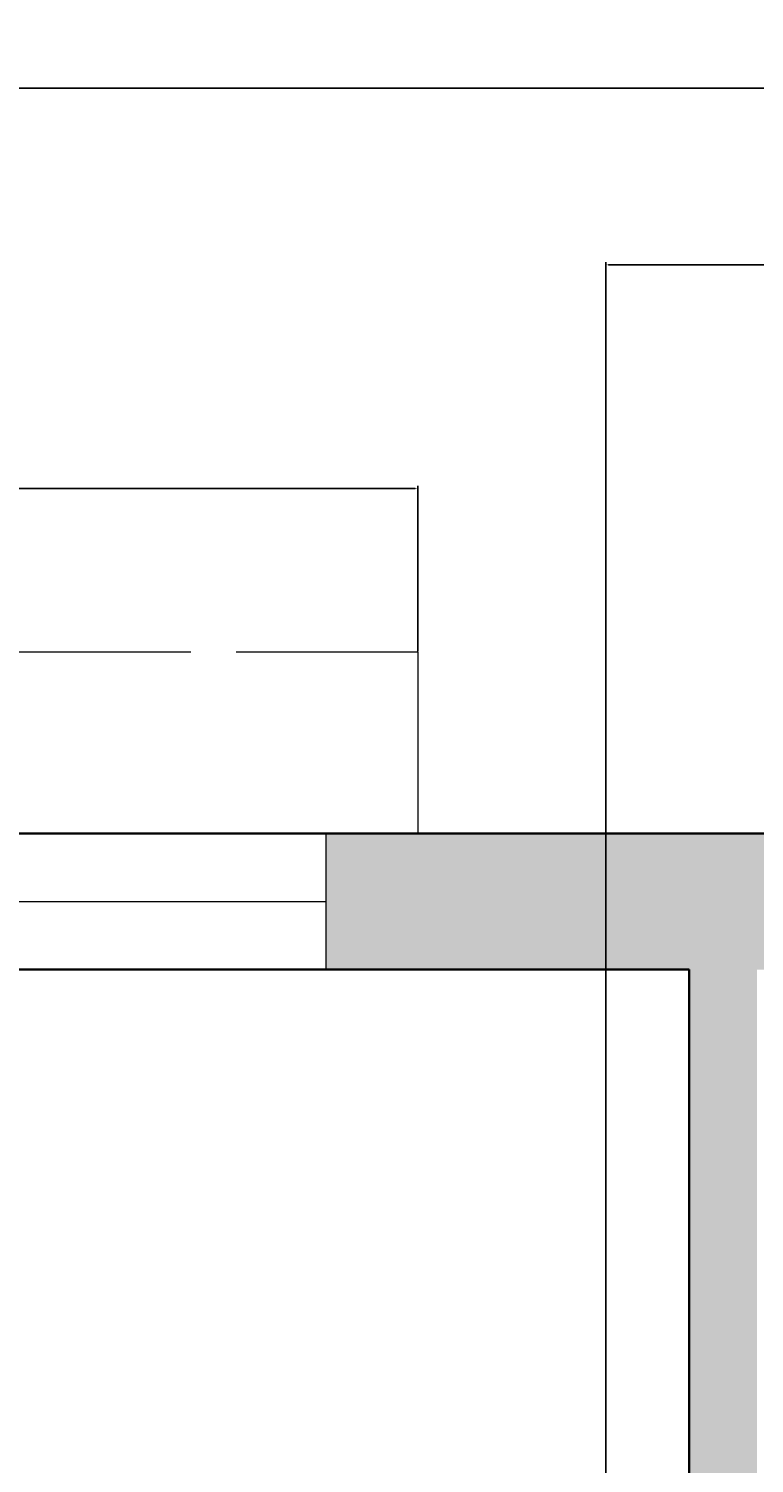
# Model space of a CAD drawing. Units: inches. Extents: x -5 to 482, y -460 to 66.
# Tile 29 of 31: x 106 to 154, y -29 to 66. Entities that reach past the tile are written whole.
import ezdxf

# ---------------------------------------------------------------- set-up
doc = ezdxf.new("R2010")
doc.units = ezdxf.units.IN
doc.header["$MEASUREMENT"] = 0
doc.linetypes.add('ACAD_ISO02W100', pattern=[15, 12, -3])
for name, color, linetype, lineweight in [('A-ANNO-DIMS', 2, 'Continuous', 18), ('A-GLAZ', 4, 'Continuous', 18), ('A-GLAZ-OVHD', 4, 'ACAD_ISO02W100', 13), ('A-WALL', 7, 'Continuous', 35), ('A-WALL-PATT', 152, 'Continuous', 13)]:
    doc.layers.add(name, color=color, linetype=linetype, lineweight=lineweight)
doc.styles.get("Standard").update_dxf_attribs({"font": 'arial.ttf'})
doc.dimstyles.get("Standard").update_dxf_attribs({"dimtxt": 0.18, "dimasz": 0.18, "dimexe": 0.18, "dimexo": 0.0625, "dimgap": 0.09, "dimtad": 0, "dimtih": 1, "dimtoh": 1, "dimdec": 0, "dimzin": 0, "dimdsep": 46, "dimlunit": 3, "dimtxsty": 'Standard', "dimcen": 0.09, "dimadec": 0, "dimazin": 0, "dimtfac": 1, "dimtdec": 0, "dimtofl": 0, "dimtmove": 0, "dimatfit": 3, "dimfxl": 1, "dimtolj": 1, "dimtzin": 0, "dimarcsym": 0})

# ---------------------------------------------------------------- blocks, each defined once
blk = doc.blocks.new('*D3')
at = {"layer": 'A-ANNO-DIMS', "color": 0, "lineweight": -2, "transparency": 16777216}
for p, q in [((32.877, 13.214), (32.877, 62.612)), ((33.057, 62.432), (221.233, 62.432)), ((430.197, 62.432), (242.02, 62.432)), ((430.377, 13.214), (430.377, 62.612))]:
    blk.add_line(p, q, dxfattribs=at)
at = {"layer": 'A-ANNO-DIMS', "color": 0, "transparency": 16777216}
for points in [[(33.057, 62.462), (33.057, 62.402), (32.877, 62.432)], [(430.197, 62.462), (430.197, 62.402), (430.377, 62.432)]]:
    blk.add_solid(points, dxfattribs=at)
at = {"layer": 'Defpoints', "color": 0, "transparency": 16777216}
for p in [(430.377, 62.432), (32.877, 13.151), (430.377, 13.151)]:
    blk.add_point(p, dxfattribs=at)
at = {"layer": 'A-ANNO-DIMS', "color": 0, "transparency": 16777216, "insert": (231.627, 62.432), "char_height": 6, "attachment_point": 5}
blk.add_mtext('\\A1;33\'-2"', dxfattribs=at)
blk = doc.blocks.new('WIN-GLAZ-60IN')
for p, q in [((0, 9), (60, 9)), ((0, 4.5), (60, 4.5)), ((60, 0), (0, 0))]:
    blk.add_line(p, q)
blk = doc.blocks.new('WIN-SHADE-72IN')
for p, q in [((0, 12), (72, 12)), ((0, 12), (0, 0)), ((72, 12), (72, 0))]:
    blk.add_line(p, q)
blk = doc.blocks.new('*D45')
at = {"layer": 'A-ANNO-DIMS', "color": 0, "lineweight": -2, "transparency": 16777216}
for p, q in [((59.948, 25.214), (59.948, 36.131)), ((131.948, 25.214), (131.948, 36.131)), ((60.128, 35.951), (94.251, 35.951)), ((131.768, 35.951), (97.645, 35.951))]:
    blk.add_line(p, q, dxfattribs=at)
at = {"layer": 'A-ANNO-DIMS', "color": 0, "transparency": 16777216}
for points in [[(60.128, 35.981), (60.128, 35.921), (59.948, 35.951)], [(131.768, 35.981), (131.768, 35.921), (131.948, 35.951)]]:
    blk.add_solid(points, dxfattribs=at)
at = {"layer": 'Defpoints', "color": 0, "transparency": 16777216}
for p in [(131.948, 35.951), (59.948, 25.151), (131.948, 25.151)]:
    blk.add_point(p, dxfattribs=at)
at = {"layer": 'A-ANNO-DIMS', "color": 0, "transparency": 16777216, "insert": (95.948, 35.951), "char_height": 0.18, "attachment_point": 5}
blk.add_mtext('\\A1;WINDOW SHADE 6\'-0" TYP.', dxfattribs=at)
blk = doc.blocks.new('*D73')
at = {"layer": 'A-ANNO-DIMS', "color": 0, "lineweight": -2, "transparency": 16777216}
for p, q in [((144.377, -295.799), (144.377, 50.931)), ((144.557, 50.751), (160.976, 50.751)), ((178.197, 50.751), (161.777, 50.751)), ((178.377, -295.799), (178.377, 50.931))]:
    blk.add_line(p, q, dxfattribs=at)
at = {"layer": 'A-ANNO-DIMS', "color": 0, "transparency": 16777216}
for points in [[(144.557, 50.781), (144.557, 50.721), (144.377, 50.751)], [(178.197, 50.781), (178.197, 50.721), (178.377, 50.751)]]:
    blk.add_solid(points, dxfattribs=at)
at = {"layer": 'Defpoints', "color": 0, "transparency": 16777216}
for p in [(178.377, 50.751), (144.377, -295.861), (178.377, -295.861)]:
    blk.add_point(p, dxfattribs=at)
at = {"layer": 'A-ANNO-DIMS', "color": 0, "transparency": 16777216, "insert": (161.377, 50.751), "char_height": 0.18, "attachment_point": 5}
blk.add_mtext('\\A1;2\'-10"', dxfattribs=at)

msp = doc.modelspace()

# ---------------------------------------------------------------- hatches: boundary and pattern name
at = {"layer": 'A-WALL-PATT'}
h = msp.add_hatch(color=256, dxfattribs=at)
h.dxf.hatch_style = 1
h.paths.add_polyline_path([(149.377, -412.849), (144.377, -412.849), (144.377, -283.849), (144.377, -279.349), (133.877, -279.349), (133.877, -283.849), (139.877, -283.849), (139.877, -412.849), (133.51, -412.849), (133.51, -413.916), (102.652, -413.916), (102.652, -421.02), (133.51, -421.02), (133.51, -421.849), (149.377, -421.849)])
h.paths.add_polyline_path([(226.054, -412.849), (218.877, -412.849), (218.877, -350.849), (262.877, -350.849), (262.877, -386.849), (267.377, -386.849), (267.377, -283.849), (270.377, -283.849), (270.377, -279.349), (244.877, -279.349), (244.877, -283.849), (262.877, -283.849), (262.877, -346.349), (218.877, -346.349), (218.877, -283.849), (220.877, -283.849), (220.877, -279.349), (214.377, -279.349), (214.377, -283.849), (214.377, -412.849), (209.377, -412.849), (209.377, -421.849), (226.054, -421.849)])
h.paths.add_polyline_path([(315.815, -412.849), (250.054, -412.849), (250.054, -421.849), (315.815, -421.849)])
h.paths.add_polyline_path([(430.377, -378.349), (421.377, -378.349), (421.377, -412.849), (375.815, -412.849), (375.815, -421.849), (430.377, -421.849)])
h.paths.add_polyline_path([(78.691, -413.916), (47.68, -413.916), (47.68, -412.849), (41.877, -412.849), (41.877, -283.849), (109.877, -283.849), (109.877, -279.349), (41.877, -279.349), (41.877, -241.849), (32.877, -241.849), (32.877, -421.849), (47.68, -421.849), (47.68, -421.02), (78.691, -421.02)])
h.paths.add_polyline_path([(41.877, -144.349), (154.377, -144.349), (154.377, -137.849), (149.877, -137.849), (149.877, -139.849), (41.877, -139.849), (41.877, -97.849), (32.877, -97.849), (32.877, -181.849), (41.877, -181.849)])
h.paths.add_polyline_path([(430.377, -241.849), (421.377, -241.849), (421.377, -279.349), (309.377, -279.349), (309.377, -170.349), (304.877, -170.349), (304.877, -279.349), (294.377, -279.349), (294.377, -283.849), (421.377, -283.849), (421.377, -318.349), (430.377, -318.349)])
h.paths.add_polyline_path([(430.377, -119.849), (421.377, -119.849), (421.377, -139.849), (419.377, -139.849), (419.377, -144.349), (421.377, -144.349), (421.377, -181.849), (430.377, -181.849)])
h.paths.add_polyline_path([(395.377, -139.849), (377.377, -139.849), (377.377, -75.849), (421.377, -75.849), (421.377, -95.849), (430.377, -95.849), (430.377, -45.599), (421.377, -45.599), (421.377, -71.349), (377.377, -71.349), (377.377, -22.849), (372.877, -22.849), (372.877, -139.849), (242.877, -139.849), (242.877, -137.849), (238.377, -137.849), (238.377, -144.349), (304.877, -144.349), (304.877, -146.349), (309.377, -146.349), (309.377, -144.349), (395.377, -144.349)])
h.paths.add_polyline_path([(65.877, 13.151), (32.877, 13.151), (32.877, -37.849), (41.877, -37.849), (41.877, 4.151), (65.877, 4.151)])
h.paths.add_polyline_path([(166.377, 13.151), (125.877, 13.151), (125.877, 4.151), (149.877, 4.151), (149.877, -113.849), (154.377, -113.849), (154.377, 4.151), (166.377, 4.151)])
h.paths.add_polyline_path([(277.877, 13.151), (226.377, 13.151), (226.377, 4.151), (238.377, 4.151), (238.377, -113.849), (242.877, -113.849), (242.877, 4.151), (277.877, 4.151)])
h.paths.add_polyline_path([(430.377, 13.151), (337.877, 13.151), (337.877, 4.151), (372.877, 4.151), (372.877, 1.151), (377.377, 1.151), (377.377, 4.151), (421.377, 4.151), (421.377, -21.599), (430.377, -21.599)])

# ---------------------------------------------------------------- linework, layer by layer
at = {"layer": 'A-GLAZ'}
msp.add_line((125.877, 13.151), (125.877, 4.151), dxfattribs=at)
at = {"layer": 'A-WALL'}
for p, q in [((32.877, 13.151), (430.377, 13.151)), ((41.877, 4.151), (149.877, 4.151)), ((149.877, 4.151), (149.877, -113.849))]:
    msp.add_line(p, q, dxfattribs=at)

# ---------------------------------------------------------------- block references
at = {"layer": 'A-GLAZ'}
msp.add_blockref('WIN-GLAZ-60IN', (65.877, 4.151), dxfattribs=at)
at = {"layer": 'A-GLAZ-OVHD'}
msp.add_blockref('WIN-SHADE-72IN', (59.948, 13.151), dxfattribs=at)

# ---------------------------------------------------------------- dimensions: what is measured, and where the dimension line sits
at = {"layer": 'A-ANNO-DIMS'}
for base, p1, p2, override, picture, middle in [((430.376735986, 62.431571932), (32.876735986, 13.151335974), (430.376735986, 13.151335974), {"dimtxt": 6, "dimclrd": 0, "dimclre": 0, "dimclrt": 0}, '*D3', (231.626735986, 62.431571932)), ((178.377, 50.751), (144.377, -295.861), (178.377, -295.861), {"dimdec": 1, "dimlfac": 1, "dimrnd": 0, "dimzin": 1, "dimdsep": 46, "dimlunit": 4, "dimfrac": 2}, '*D73', (161.377, 50.751))]:
    dim = msp.add_linear_dim(base=base, p1=p1, p2=p2, dimstyle='Standard', override=override, dxfattribs=at)
    dim.commit()
    dim.dimension.update_dxf_attribs({"geometry": picture, "text_midpoint": middle})
dim = msp.add_linear_dim(base=(131.948, 35.951), p1=(59.948, 25.151), p2=(131.948, 25.151), text='WINDOW SHADE <> TYP.', dimstyle='Standard', override={"dimdec": 1, "dimlfac": 1, "dimrnd": 0, "dimzin": 1, "dimdsep": 46, "dimlunit": 4, "dimfrac": 2}, dxfattribs=at)
dim.commit()
dim.dimension.update_dxf_attribs({"geometry": '*D45', "text_midpoint": (95.948, 35.951)})

doc.saveas('drawing.dxf')
